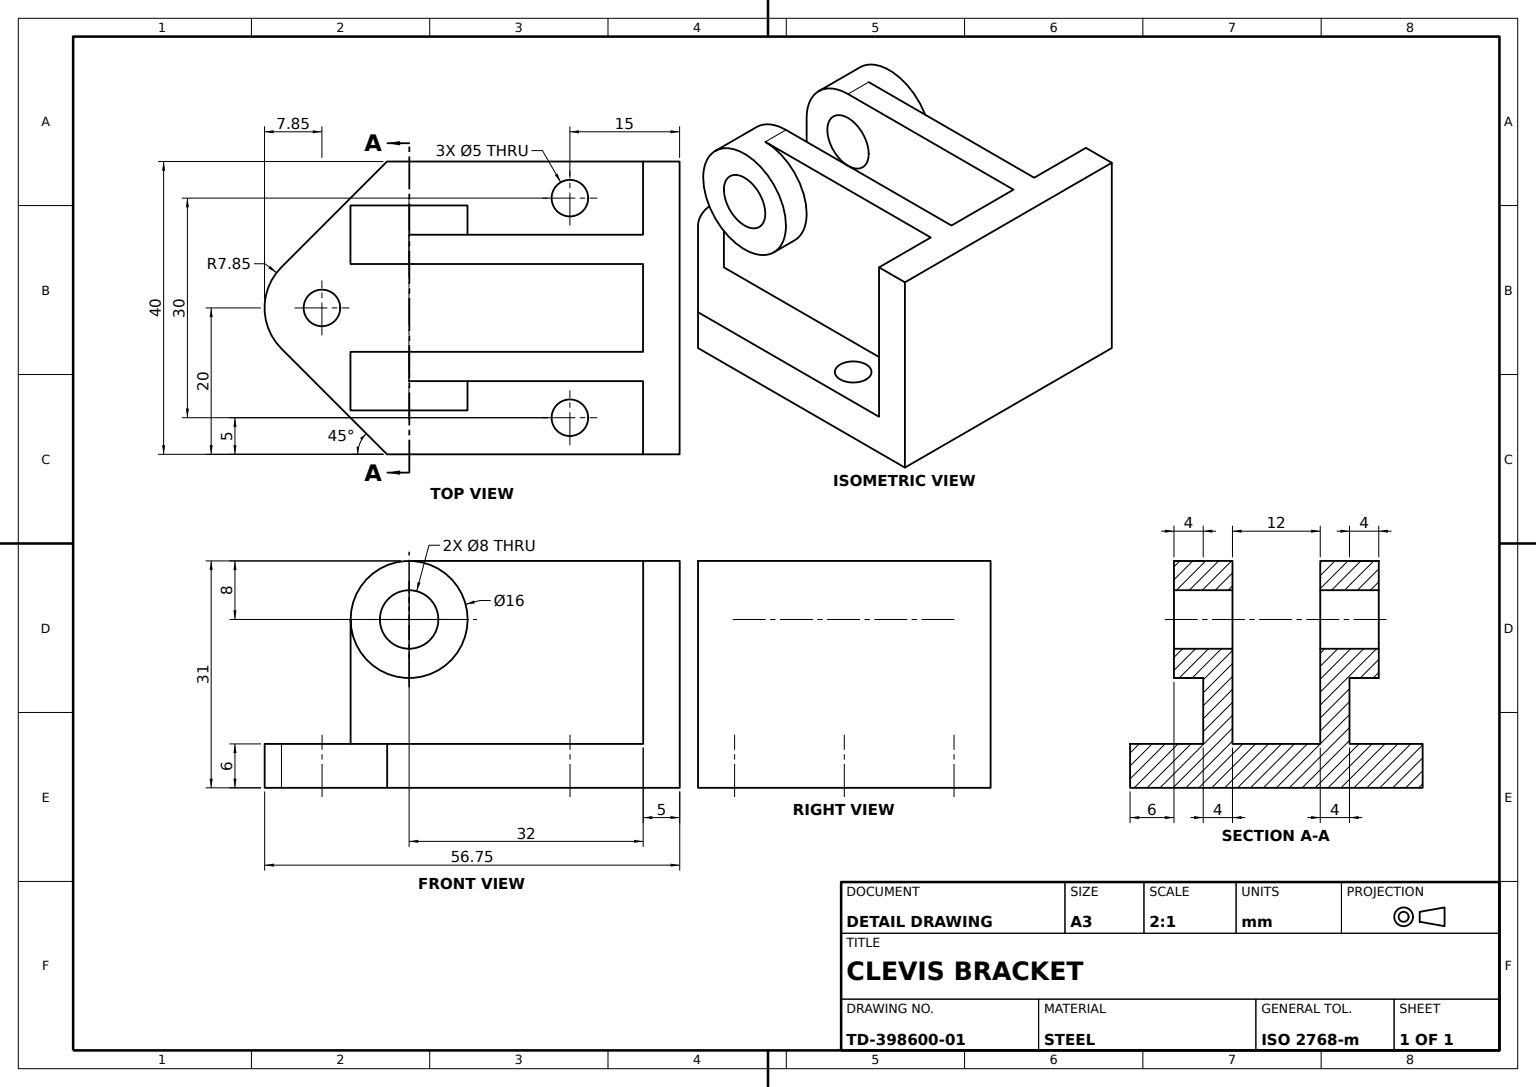
from build123d import *

# Parameters (mm, degrees)
BASE_PLATE_SKETCH_R             = 2.5
POINTED_BASE_PLATE_DEPTH        = 6
BACK_WALL_AND_CLEVIS_LUGS_DEPTH = 25
LUG_BOSS_SKETCH_R               = 8
LUG_BOSS_SKETCH_R_2             = 4
LUG_BOSS_DEPTH                  = 4
PIN_HOLE_REACH                  = 75.058
PIN_HOLE_SKETCH_R               = 4
BASE_MOUNTING_HOLES_REACH       = 67.158
MOUNTING_HOLES_SKETCH_R         = 2.5


with BuildPart() as part:
    # Base Plate Sketch → Pointed Base Plate (new body)
    with BuildSketch(Plane(origin=(0, 0, 0), x_dir=(1, 0, 0), z_dir=(0, 1, 0))):
        with BuildLine():
            Line((-20, 0), (20, 0))
            Line((20, 0), (20, -40))
            Line((20, -40), (5.548667415, -54.451332585))
            ThreePointArc((5.548667415, -54.451332585), (0, -56.749665881), (-5.548667415, -54.451332585))
            Line((-5.548667415, -54.451332585), (-20, -40))
            Line((-20, -40), (-20, 0))
        make_face()
        with Locations(Location((0, -48.902665169, 0), (0, 0, 270))):
            Circle(BASE_PLATE_SKETCH_R, mode=Mode.SUBTRACT)
    extrude(amount=POINTED_BASE_PLATE_DEPTH)

    # Back Wall and Lugs Sketch → Back Wall and Clevis Lugs (add)
    with BuildSketch(Plane(origin=(0, 6, 0), x_dir=(1, 0, 0), z_dir=(0, 1, 0))):
        Polygon((-20, 0), (20, 0), (20, -5), (10, -5), (10, -45), (6, -45), (6, -5), (-6, -5), (-6, -45), (-10, -45), (-10, -5), (-20, -5), align=None)
    extrude(amount=BACK_WALL_AND_CLEVIS_LUGS_DEPTH)

    # Lug Boss Sketch → Lug Boss (add)
    with BuildSketch(Plane(origin=(10, 0, 0), x_dir=(0, 0, -1), z_dir=(1, 0, 0))):
        with Locations(Location((-37, 23, 0), (0, 0, 180))):
            Circle(LUG_BOSS_SKETCH_R)
        with Locations((-37, 23)):
            Circle(LUG_BOSS_SKETCH_R_2, mode=Mode.SUBTRACT)
    lug_boss = extrude(amount=LUG_BOSS_DEPTH)

    # Pin Hole Sketch → Pin Hole (cut, up to next)
    with BuildSketch(Plane(origin=(14, 0, 0), x_dir=(0, 0, -1), z_dir=(1, 0, 0)), mode=Mode.PRIVATE) as pin_hole_sk1:
        with Locations((-37, 23)):
            Circle(PIN_HOLE_SKETCH_R)
    pin_hole_tool1 = extrude(pin_hole_sk1.sketch, amount=-PIN_HOLE_REACH, mode=Mode.PRIVATE) & part.part
    # Pin Hole Sketch → Pin Hole (cut, up to next)
    with BuildSketch(Plane(origin=(14, 0, 0), x_dir=(0, 0, -1), z_dir=(1, 0, 0)), mode=Mode.PRIVATE) as pin_hole_sk2:
        with BuildLine():
            Line((-45, 31), (-45, 23))
            ThreePointArc((-45, 23), (-42.656854249, 28.656854249), (-37, 31))
            Line((-37, 31), (-45, 31))
        make_face()
    pin_hole_tool2 = extrude(pin_hole_sk2.sketch, amount=-PIN_HOLE_REACH, mode=Mode.PRIVATE) & part.part
    pin_hole_1 = pin_hole_tool1.solids().sort_by_distance((14, 23, 37))[0]
    add(pin_hole_1, mode=Mode.SUBTRACT)
    pin_hole_2 = pin_hole_tool2.solids().sort_by_distance((14, 29.213056, 43.213056))[0]
    add(pin_hole_2, mode=Mode.SUBTRACT)
    pin_hole = pin_hole_1 + pin_hole_2  # Pin Hole as one shape, for the pattern or mirror that repeats it

    # Lug Boss and Pin Hole Mirror: Lug Boss, Pin Hole across plane
    add(lug_boss.mirror(Plane(origin=(0, 0, 0), x_dir=(0, 0, 1), z_dir=(1, 0, 0))))
    add(pin_hole.mirror(Plane(origin=(0, 0, 0), x_dir=(0, 0, 1), z_dir=(1, 0, 0))), mode=Mode.SUBTRACT)

    # Mounting Holes Sketch → Base Mounting Holes (cut, up to next)
    with BuildSketch(Plane(origin=(0, 6, 0), x_dir=(1, 0, 0), z_dir=(0, 1, 0)), mode=Mode.PRIVATE) as base_mounting_holes_sk1:
        with Locations(Location((-15, -15, 0), (0, 0, 270))):
            Circle(MOUNTING_HOLES_SKETCH_R)
    base_mounting_holes_tool1 = extrude(base_mounting_holes_sk1.sketch, amount=-BASE_MOUNTING_HOLES_REACH, mode=Mode.PRIVATE) & part.part
    # Mounting Holes Sketch → Base Mounting Holes (cut, up to next)
    with BuildSketch(Plane(origin=(0, 6, 0), x_dir=(1, 0, 0), z_dir=(0, 1, 0)), mode=Mode.PRIVATE) as base_mounting_holes_sk2:
        with Locations(Location((15, -15, 0), (0, 0, 270))):
            Circle(MOUNTING_HOLES_SKETCH_R)
    base_mounting_holes_tool2 = extrude(base_mounting_holes_sk2.sketch, amount=-BASE_MOUNTING_HOLES_REACH, mode=Mode.PRIVATE) & part.part
    add(base_mounting_holes_tool1.solids().sort_by_distance((-15, 6, 15))[0], mode=Mode.SUBTRACT)
    add(base_mounting_holes_tool2.solids().sort_by_distance((15, 6, 15))[0], mode=Mode.SUBTRACT)


solid = part.part
